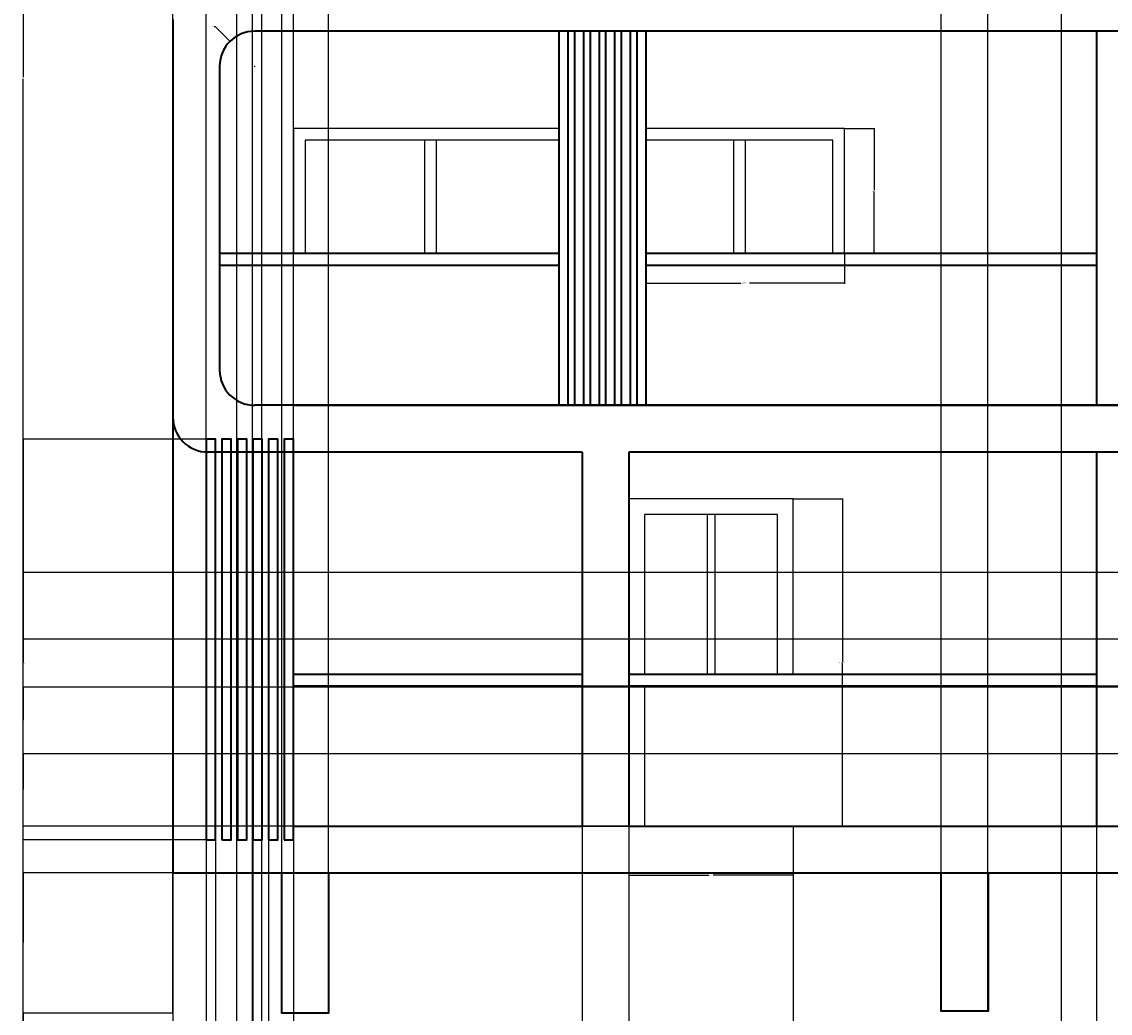
# Model space of a CAD drawing. Units: inches. Extents: x -15 to 605, y -220 to 570.
# Tile 2 of 10: x -15 to 265, y -32 to 222. Entities that reach past the tile are written whole.
import ezdxf

# ---------------------------------------------------------------- set-up
doc = ezdxf.new("R2010")
doc.units = ezdxf.units.IN
doc.header["$MEASUREMENT"] = 0
for name, color, linetype, lineweight in [('A-ANNO-DIMS', 2, 'Continuous', 18), ('A-COLS', 7, 'Continuous', 35), ('A-DOOR', 4, 'Continuous', 25), ('A-ELEV', 7, 'Continuous', 35), ('A-GLAZ', 4, 'Continuous', 25)]:
    doc.layers.add(name, color=color, linetype=linetype, lineweight=lineweight)
doc.styles.get("Standard").update_dxf_attribs({"font": 'arial.ttf'})
doc.dimstyles.get("Standard").update_dxf_attribs({"dimtxt": 0.18, "dimasz": 0.18, "dimexe": 0.18, "dimexo": 0.0625, "dimgap": 0.09, "dimtad": 0, "dimtih": 1, "dimtoh": 1, "dimdec": 4, "dimzin": 0, "dimdsep": 46, "dimtxsty": 'Standard', "dimcen": 0.09, "dimadec": 0, "dimazin": 0, "dimtfac": 1, "dimtdec": 4, "dimtofl": 0, "dimtmove": 0, "dimatfit": 3, "dimfxl": 1, "dimtolj": 1, "dimtzin": 0, "dimarcsym": 0})

# ---------------------------------------------------------------- blocks, each defined once
blk = doc.blocks.new('DOOR-ELEV')
for p, q in [((20.09, 80), (20.09, 39)), ((22.09, 80), (22.09, 39))]:
    blk.add_line(p, q)
for points in [[(42.18, 39), (42.18, 84), (0, 84), (0, 0), (42.18, 0)], [(38.18, 39), (38.18, 80), (4, 80), (4, 39)], [(4, 36), (4, 0)]]:
    blk.add_lwpolyline(points)
blk = doc.blocks.new('WIN-ELEV')
for p, q in [((22.41, 29.07), (22.41, 0)), ((25.41, 29.07), (25.41, 0))]:
    blk.add_line(p, q)
for points in [[(50.87, 0), (50.87, 32.07), (0, 32.07)], [(47.87, 0), (47.87, 29.07), (0, 29.07)]]:
    blk.add_lwpolyline(points)
blk = doc.blocks.new('*D3')
at = {"layer": 'A-ANNO-DIMS', "color": 0, "lineweight": -2, "transparency": 16777216}
for p, q in [((183.23, 99.82), (195.95, 99.82)), ((195.77, 99.64), (195.77, 58)), ((195.77, 16), (195.77, 57.64)), ((183.23, 15.82), (195.95, 15.82))]:
    blk.add_line(p, q, dxfattribs=at)
at = {"layer": 'A-ANNO-DIMS', "color": 0, "transparency": 16777216}
for points in [[(195.74, 99.64), (195.8, 99.64), (195.77, 99.82)], [(195.74, 16), (195.8, 16), (195.77, 15.82)]]:
    blk.add_solid(points, dxfattribs=at)
at = {"layer": 'Defpoints', "color": 0, "transparency": 16777216}
for p in [(183.17, 99.82), (195.77, 99.82), (183.17, 15.82)]:
    blk.add_point(p, dxfattribs=at)
at = {"layer": 'A-ANNO-DIMS', "color": 0, "transparency": 16777216, "insert": (195.77, 57.82), "char_height": 0.18, "attachment_point": 5}
blk.add_mtext('\\A1;DOOR 84 TYP.', dxfattribs=at)
blk = doc.blocks.new('*D4')
at = {"layer": 'A-ANNO-DIMS', "color": 0, "lineweight": -2, "transparency": 16777216}
for p, q in [((140.99, 15.76), (140.99, 3.04)), ((183.17, 15.76), (183.17, 3.04)), ((141.17, 3.22), (161.55, 3.22)), ((182.99, 3.22), (162.61, 3.22))]:
    blk.add_line(p, q, dxfattribs=at)
at = {"layer": 'A-ANNO-DIMS', "color": 0, "transparency": 16777216}
for points in [[(141.17, 3.25), (141.17, 3.19), (140.99, 3.22)], [(182.99, 3.25), (182.99, 3.19), (183.17, 3.22)]]:
    blk.add_solid(points, dxfattribs=at)
at = {"layer": 'Defpoints', "color": 0, "transparency": 16777216}
for p in [(140.99, 15.82), (183.17, 15.82), (183.17, 3.22)]:
    blk.add_point(p, dxfattribs=at)
at = {"layer": 'A-ANNO-DIMS', "color": 0, "transparency": 16777216, "insert": (162.08, 3.22), "char_height": 0.18, "attachment_point": 5}
blk.add_mtext('\\A1;42 TYP.', dxfattribs=at)
blk = doc.blocks.new('*D5')
at = {"layer": 'A-ANNO-DIMS', "color": 0, "lineweight": -2, "transparency": 16777216}
for p, q in [((145.43, 162.76), (145.43, 155.01)), ((196.29, 162.76), (196.29, 155.01)), ((145.61, 155.19), (169.74, 155.19)), ((196.11, 155.19), (171.98, 155.19))]:
    blk.add_line(p, q, dxfattribs=at)
at = {"layer": 'A-ANNO-DIMS', "color": 0, "transparency": 16777216}
for points in [[(145.61, 155.22), (145.61, 155.16), (145.43, 155.19)], [(196.11, 155.22), (196.11, 155.16), (196.29, 155.19)]]:
    blk.add_solid(points, dxfattribs=at)
at = {"layer": 'Defpoints', "color": 0, "transparency": 16777216}
for p in [(145.43, 162.82), (196.29, 162.82), (196.29, 155.19)]:
    blk.add_point(p, dxfattribs=at)
at = {"layer": 'A-ANNO-DIMS', "color": 0, "transparency": 16777216, "insert": (170.86, 155.19), "char_height": 0.18, "attachment_point": 5}
blk.add_mtext('\\A1;WINDOW 51 TYP.', dxfattribs=at)
blk = doc.blocks.new('*D6')
at = {"layer": 'A-ANNO-DIMS', "color": 0, "lineweight": -2, "transparency": 16777216}
for p, q in [((196.36, 194.89), (204.1, 194.89)), ((203.92, 194.71), (203.92, 179.04)), ((203.92, 163), (203.92, 178.67)), ((196.36, 162.82), (204.1, 162.82))]:
    blk.add_line(p, q, dxfattribs=at)
at = {"layer": 'A-ANNO-DIMS', "color": 0, "transparency": 16777216}
for points in [[(203.89, 194.71), (203.95, 194.71), (203.92, 194.89)], [(203.89, 163), (203.95, 163), (203.92, 162.82)]]:
    blk.add_solid(points, dxfattribs=at)
at = {"layer": 'Defpoints', "color": 0, "transparency": 16777216}
for p in [(196.29, 194.89), (203.92, 194.89), (196.29, 162.82)]:
    blk.add_point(p, dxfattribs=at)
at = {"layer": 'A-ANNO-DIMS', "color": 0, "transparency": 16777216, "insert": (203.92, 178.85), "char_height": 0.18, "attachment_point": 5}
blk.add_mtext('\\A1;32 TYP.', dxfattribs=at)
blk = doc.blocks.new('*D7')
at = {"layer": 'A-ANNO-DIMS', "color": 0, "lineweight": -2, "transparency": 16777216}
for p, q in [((23.99, 3.76), (23.99, -154.76)), ((566.72, -116.24), (566.72, -154.76)), ((24.17, -154.58), (294.96, -154.58)), ((566.54, -154.58), (295.75, -154.58))]:
    blk.add_line(p, q, dxfattribs=at)
at = {"layer": 'A-ANNO-DIMS', "color": 0, "transparency": 16777216}
for points in [[(24.17, -154.55), (24.17, -154.61), (23.99, -154.58)], [(566.54, -154.55), (566.54, -154.61), (566.72, -154.58)]]:
    blk.add_solid(points, dxfattribs=at)
at = {"layer": 'Defpoints', "color": 0, "transparency": 16777216}
for p in [(23.99, 3.82), (566.72, -116.18), (566.72, -154.58)]:
    blk.add_point(p, dxfattribs=at)
at = {"layer": 'A-ANNO-DIMS', "color": 0, "transparency": 16777216, "insert": (295.35, -154.58), "char_height": 0.18, "attachment_point": 5}
blk.add_mtext('\\A1;542.7', dxfattribs=at)
blk = doc.blocks.new('*D8')
at = {"layer": 'A-ANNO-DIMS', "color": 0, "lineweight": -2, "transparency": 16777216}
for p, q in [((23.99, 3.88), (23.99, 570.4)), ((24.17, 570.22), (263.7, 570.22)), ((503.81, 570.22), (264.28, 570.22)), ((503.99, 531.88), (503.99, 570.4))]:
    blk.add_line(p, q, dxfattribs=at)
at = {"layer": 'A-ANNO-DIMS', "color": 0, "transparency": 16777216}
for points in [[(24.17, 570.25), (24.17, 570.19), (23.99, 570.22)], [(503.81, 570.25), (503.81, 570.19), (503.99, 570.22)]]:
    blk.add_solid(points, dxfattribs=at)
at = {"layer": 'Defpoints', "color": 0, "transparency": 16777216}
for p in [(503.99, 570.22), (503.99, 531.82), (23.99, 3.82)]:
    blk.add_point(p, dxfattribs=at)
at = {"layer": 'A-ANNO-DIMS', "color": 0, "transparency": 16777216, "insert": (263.99, 570.22), "char_height": 0.18, "attachment_point": 5}
blk.add_mtext('\\A1;480', dxfattribs=at)
blk = doc.blocks.new('*D9')
at = {"layer": 'A-ANNO-DIMS', "color": 0, "lineweight": -2, "transparency": 16777216}
for p, q in [((503.92, 531.82), (-14.59, 531.82)), ((-14.41, 531.64), (-14.41, 208)), ((-14.41, -116), (-14.41, 207.64)), ((23.92, -116.18), (-14.59, -116.18))]:
    blk.add_line(p, q, dxfattribs=at)
at = {"layer": 'A-ANNO-DIMS', "color": 0, "transparency": 16777216}
for points in [[(-14.44, 531.64), (-14.38, 531.64), (-14.41, 531.82)], [(-14.44, -116), (-14.38, -116), (-14.41, -116.18)]]:
    blk.add_solid(points, dxfattribs=at)
at = {"layer": 'Defpoints', "color": 0, "transparency": 16777216}
for p in [(-14.41, 531.82), (503.99, 531.82), (23.99, -116.18)]:
    blk.add_point(p, dxfattribs=at)
at = {"layer": 'A-ANNO-DIMS', "color": 0, "transparency": 16777216, "insert": (-14.41, 207.82), "char_height": 0.18, "attachment_point": 5}
blk.add_mtext('\\A1;648', dxfattribs=at)
blk = doc.blocks.new('*D18')
at = {"layer": 'A-ANNO-DIMS', "color": 0, "lineweight": -2, "transparency": 16777216}
for p, q in [((23.99, 3.88), (23.99, 570.4)), ((24.17, 570.22), (143.44, 570.22)), ((263.64, 570.22), (144.37, 570.22)), ((263.82, 447.88), (263.82, 570.4))]:
    blk.add_line(p, q, dxfattribs=at)
at = {"layer": 'A-ANNO-DIMS', "color": 0, "transparency": 16777216}
for points in [[(24.17, 570.25), (24.17, 570.19), (23.99, 570.22)], [(263.64, 570.25), (263.64, 570.19), (263.82, 570.22)]]:
    blk.add_solid(points, dxfattribs=at)
at = {"layer": 'Defpoints', "color": 0, "transparency": 16777216}
for p in [(263.82, 570.22), (263.82, 447.82), (23.99, 3.82)]:
    blk.add_point(p, dxfattribs=at)
at = {"layer": 'A-ANNO-DIMS', "color": 0, "transparency": 16777216, "insert": (143.9, 570.22), "char_height": 0.18, "attachment_point": 5}
blk.add_mtext('\\A1;239.83', dxfattribs=at)
blk = doc.blocks.new('*D21')
at = {"layer": 'A-ANNO-DIMS', "color": 0, "lineweight": -2, "transparency": 16777216}
for p, q in [((23.92, 3.82), (-14.59, 3.82)), ((-14.41, 3.64), (-14.41, -14)), ((-14.41, -32), (-14.41, -14.36)), ((23.92, -32.18), (-14.59, -32.18))]:
    blk.add_line(p, q, dxfattribs=at)
at = {"layer": 'A-ANNO-DIMS', "color": 0, "transparency": 16777216}
for points in [[(-14.44, 3.64), (-14.38, 3.64), (-14.41, 3.82)], [(-14.44, -32), (-14.38, -32), (-14.41, -32.18)]]:
    blk.add_solid(points, dxfattribs=at)
at = {"layer": 'Defpoints', "color": 0, "transparency": 16777216}
for p in [(-14.41, 3.82), (23.99, 3.82), (23.99, -32.18)]:
    blk.add_point(p, dxfattribs=at)
at = {"layer": 'A-ANNO-DIMS', "color": 0, "transparency": 16777216, "insert": (-14.41, -14.18), "char_height": 0.18, "attachment_point": 5}
blk.add_mtext('\\A1;36', dxfattribs=at)
blk = doc.blocks.new('*D23')
at = {"layer": 'A-ANNO-DIMS', "color": 0, "lineweight": -2, "transparency": 16777216}
for p, q in [((54.93, 15.76), (54.93, -154.76)), ((23.99, 3.76), (23.99, -154.76)), ((24.17, -154.58), (39, -154.58)), ((54.75, -154.58), (39.92, -154.58))]:
    blk.add_line(p, q, dxfattribs=at)
at = {"layer": 'A-ANNO-DIMS', "color": 0, "transparency": 16777216}
for points in [[(24.17, -154.55), (24.17, -154.61), (23.99, -154.58)], [(54.75, -154.55), (54.75, -154.61), (54.93, -154.58)]]:
    blk.add_solid(points, dxfattribs=at)
at = {"layer": 'Defpoints', "color": 0, "transparency": 16777216}
for p in [(54.93, 15.82), (23.99, 3.82), (54.93, -154.58)]:
    blk.add_point(p, dxfattribs=at)
at = {"layer": 'A-ANNO-DIMS', "color": 0, "transparency": 16777216, "insert": (39.46, -154.58), "char_height": 0.18, "attachment_point": 5}
blk.add_mtext('\\A1;30.946', dxfattribs=at)
blk = doc.blocks.new('*D24')
at = {"layer": 'A-ANNO-DIMS', "color": 0, "lineweight": -2, "transparency": 16777216}
for p, q in [((54.93, 15.76), (54.93, -154.76)), ((128.99, 15.76), (128.99, -154.76)), ((55.11, -154.58), (91.57, -154.58)), ((128.81, -154.58), (92.35, -154.58))]:
    blk.add_line(p, q, dxfattribs=at)
at = {"layer": 'A-ANNO-DIMS', "color": 0, "transparency": 16777216}
for points in [[(55.11, -154.55), (55.11, -154.61), (54.93, -154.58)], [(128.81, -154.55), (128.81, -154.61), (128.99, -154.58)]]:
    blk.add_solid(points, dxfattribs=at)
at = {"layer": 'Defpoints', "color": 0, "transparency": 16777216}
for p in [(54.93, 15.82), (128.99, 15.82), (128.99, -154.58)]:
    blk.add_point(p, dxfattribs=at)
at = {"layer": 'A-ANNO-DIMS', "color": 0, "transparency": 16777216, "insert": (91.96, -154.58), "char_height": 0.18, "attachment_point": 5}
blk.add_mtext('\\A1;74.05', dxfattribs=at)
blk = doc.blocks.new('*D25')
at = {"layer": 'A-ANNO-DIMS', "color": 0, "lineweight": -2, "transparency": 16777216}
for p, q in [((128.99, 15.76), (128.99, -154.76)), ((140.99, 15.76), (140.99, -154.76)), ((129.17, -154.58), (134.78, -154.58)), ((140.81, -154.58), (135.2, -154.58))]:
    blk.add_line(p, q, dxfattribs=at)
at = {"layer": 'A-ANNO-DIMS', "color": 0, "transparency": 16777216}
for points in [[(129.17, -154.55), (129.17, -154.61), (128.99, -154.58)], [(140.81, -154.55), (140.81, -154.61), (140.99, -154.58)]]:
    blk.add_solid(points, dxfattribs=at)
at = {"layer": 'Defpoints', "color": 0, "transparency": 16777216}
for p in [(128.99, 15.82), (140.99, 15.82), (140.99, -154.58)]:
    blk.add_point(p, dxfattribs=at)
at = {"layer": 'A-ANNO-DIMS', "color": 0, "transparency": 16777216, "insert": (134.99, -154.58), "char_height": 0.18, "attachment_point": 5}
blk.add_mtext('\\A1;12', dxfattribs=at)
blk = doc.blocks.new('*D26')
at = {"layer": 'A-ANNO-DIMS', "color": 0, "lineweight": -2, "transparency": 16777216}
for p, q in [((140.99, 15.76), (140.99, -154.76)), ((183.17, 15.76), (183.17, -154.76)), ((141.17, -154.58), (161.68, -154.58)), ((182.99, -154.58), (162.48, -154.58))]:
    blk.add_line(p, q, dxfattribs=at)
at = {"layer": 'A-ANNO-DIMS', "color": 0, "transparency": 16777216}
for points in [[(141.17, -154.55), (141.17, -154.61), (140.99, -154.58)], [(182.99, -154.55), (182.99, -154.61), (183.17, -154.58)]]:
    blk.add_solid(points, dxfattribs=at)
at = {"layer": 'Defpoints', "color": 0, "transparency": 16777216}
for p in [(140.99, 15.82), (183.17, 15.82), (183.17, -154.58)]:
    blk.add_point(p, dxfattribs=at)
at = {"layer": 'A-ANNO-DIMS', "color": 0, "transparency": 16777216, "insert": (162.08, -154.58), "char_height": 0.18, "attachment_point": 5}
blk.add_mtext('\\A1;42.18', dxfattribs=at)
blk = doc.blocks.new('*D27')
at = {"layer": 'A-ANNO-DIMS', "color": 0, "lineweight": -2, "transparency": 16777216}
for p, q in [((183.17, 15.76), (183.17, -154.76)), ((260.99, 15.76), (260.99, -154.76)), ((183.35, -154.58), (221.69, -154.58)), ((260.81, -154.58), (222.47, -154.58))]:
    blk.add_line(p, q, dxfattribs=at)
at = {"layer": 'A-ANNO-DIMS', "color": 0, "transparency": 16777216}
for points in [[(183.35, -154.55), (183.35, -154.61), (183.17, -154.58)], [(260.81, -154.55), (260.81, -154.61), (260.99, -154.58)]]:
    blk.add_solid(points, dxfattribs=at)
at = {"layer": 'Defpoints', "color": 0, "transparency": 16777216}
for p in [(183.17, 15.82), (260.99, 15.82), (260.99, -154.58)]:
    blk.add_point(p, dxfattribs=at)
at = {"layer": 'A-ANNO-DIMS', "color": 0, "transparency": 16777216, "insert": (222.08, -154.58), "char_height": 0.18, "attachment_point": 5}
blk.add_mtext('\\A1;77.82', dxfattribs=at)
blk = doc.blocks.new('*D28')
at = {"layer": 'A-ANNO-DIMS', "color": 0, "lineweight": -2, "transparency": 16777216}
for p, q in [((260.99, 15.76), (260.99, -154.76)), ((272.99, 15.76), (272.99, -154.76)), ((261.17, -154.58), (266.78, -154.58)), ((272.81, -154.58), (267.2, -154.58))]:
    blk.add_line(p, q, dxfattribs=at)
at = {"layer": 'A-ANNO-DIMS', "color": 0, "transparency": 16777216}
for points in [[(261.17, -154.55), (261.17, -154.61), (260.99, -154.58)], [(272.81, -154.55), (272.81, -154.61), (272.99, -154.58)]]:
    blk.add_solid(points, dxfattribs=at)
at = {"layer": 'Defpoints', "color": 0, "transparency": 16777216}
for p in [(260.99, 15.82), (272.99, 15.82), (272.99, -154.58)]:
    blk.add_point(p, dxfattribs=at)
at = {"layer": 'A-ANNO-DIMS', "color": 0, "transparency": 16777216, "insert": (266.99, -154.58), "char_height": 0.18, "attachment_point": 5}
blk.add_mtext('\\A1;12', dxfattribs=at)
blk = doc.blocks.new('*D33')
at = {"layer": 'A-ANNO-DIMS', "color": 0, "lineweight": -2, "transparency": 16777216}
for p, q in [((491.92, 34.38), (-14.59, 34.38)), ((-14.41, 34.2), (-14.41, 25.28)), ((-14.41, 16), (-14.41, 24.92)), ((491.92, 15.82), (-14.59, 15.82))]:
    blk.add_line(p, q, dxfattribs=at)
at = {"layer": 'A-ANNO-DIMS', "color": 0, "transparency": 16777216}
for points in [[(-14.44, 34.2), (-14.38, 34.2), (-14.41, 34.38)], [(-14.44, 16), (-14.38, 16), (-14.41, 15.82)]]:
    blk.add_solid(points, dxfattribs=at)
at = {"layer": 'Defpoints', "color": 0, "transparency": 16777216}
for p in [(-14.41, 34.38), (491.99, 34.38), (491.99, 15.82)]:
    blk.add_point(p, dxfattribs=at)
at = {"layer": 'A-ANNO-DIMS', "color": 0, "transparency": 16777216, "insert": (-14.41, 25.1), "char_height": 0.18, "attachment_point": 5}
blk.add_mtext('\\A1;18.557', dxfattribs=at)
blk = doc.blocks.new('*D34')
at = {"layer": 'A-ANNO-DIMS', "color": 0, "lineweight": -2, "transparency": 16777216}
for p, q in [((491.92, 51.48), (-14.59, 51.48)), ((-14.41, 51.3), (-14.41, 43.11)), ((-14.41, 34.56), (-14.41, 42.75)), ((491.92, 34.38), (-14.59, 34.38))]:
    blk.add_line(p, q, dxfattribs=at)
at = {"layer": 'A-ANNO-DIMS', "color": 0, "transparency": 16777216}
for points in [[(-14.44, 51.3), (-14.38, 51.3), (-14.41, 51.48)], [(-14.44, 34.56), (-14.38, 34.56), (-14.41, 34.38)]]:
    blk.add_solid(points, dxfattribs=at)
at = {"layer": 'Defpoints', "color": 0, "transparency": 16777216}
for p in [(-14.41, 51.48), (491.99, 51.48), (491.99, 34.38)]:
    blk.add_point(p, dxfattribs=at)
at = {"layer": 'A-ANNO-DIMS', "color": 0, "transparency": 16777216, "insert": (-14.41, 42.93), "char_height": 0.18, "attachment_point": 5}
blk.add_mtext('\\A1;17.1', dxfattribs=at)
blk = doc.blocks.new('*D35')
at = {"layer": 'A-ANNO-DIMS', "color": 0, "lineweight": -2, "transparency": 16777216}
for p, q in [((491.92, 63.82), (-14.59, 63.82)), ((-14.41, 63.64), (-14.41, 57.83)), ((-14.41, 51.66), (-14.41, 57.47)), ((491.92, 51.48), (-14.59, 51.48))]:
    blk.add_line(p, q, dxfattribs=at)
at = {"layer": 'A-ANNO-DIMS', "color": 0, "transparency": 16777216}
for points in [[(-14.44, 63.64), (-14.38, 63.64), (-14.41, 63.82)], [(-14.44, 51.66), (-14.38, 51.66), (-14.41, 51.48)]]:
    blk.add_solid(points, dxfattribs=at)
at = {"layer": 'Defpoints', "color": 0, "transparency": 16777216}
for p in [(-14.41, 63.82), (491.99, 63.82), (491.99, 51.48)]:
    blk.add_point(p, dxfattribs=at)
at = {"layer": 'A-ANNO-DIMS', "color": 0, "transparency": 16777216, "insert": (-14.41, 57.65), "char_height": 0.18, "attachment_point": 5}
blk.add_mtext('\\A1;12.342', dxfattribs=at)
blk = doc.blocks.new('*D36')
at = {"layer": 'A-ANNO-DIMS', "color": 0, "lineweight": -2, "transparency": 16777216}
for p, q in [((491.92, 80.92), (-14.59, 80.92)), ((-14.41, 80.74), (-14.41, 72.55)), ((-14.41, 64), (-14.41, 72.19)), ((491.92, 63.82), (-14.59, 63.82))]:
    blk.add_line(p, q, dxfattribs=at)
at = {"layer": 'A-ANNO-DIMS', "color": 0, "transparency": 16777216}
for points in [[(-14.44, 80.74), (-14.38, 80.74), (-14.41, 80.92)], [(-14.44, 64), (-14.38, 64), (-14.41, 63.82)]]:
    blk.add_solid(points, dxfattribs=at)
at = {"layer": 'Defpoints', "color": 0, "transparency": 16777216}
for p in [(-14.41, 80.92), (491.99, 80.92), (491.99, 63.82)]:
    blk.add_point(p, dxfattribs=at)
at = {"layer": 'A-ANNO-DIMS', "color": 0, "transparency": 16777216, "insert": (-14.41, 72.37), "char_height": 0.18, "attachment_point": 5}
blk.add_mtext('\\A1;17.1', dxfattribs=at)
blk = doc.blocks.new('*D37')
at = {"layer": 'A-ANNO-DIMS', "color": 0, "lineweight": -2, "transparency": 16777216}
for p, q in [((129.05, 51.82), (605.3, 51.82)), ((605.12, 51.64), (605.12, 34)), ((605.12, 16), (605.12, 33.64)), ((129.05, 15.82), (605.3, 15.82))]:
    blk.add_line(p, q, dxfattribs=at)
at = {"layer": 'A-ANNO-DIMS', "color": 0, "transparency": 16777216}
for points in [[(605.09, 51.64), (605.15, 51.64), (605.12, 51.82)], [(605.09, 16), (605.15, 16), (605.12, 15.82)]]:
    blk.add_solid(points, dxfattribs=at)
at = {"layer": 'Defpoints', "color": 0, "transparency": 16777216}
for p in [(128.99, 51.82), (605.12, 51.82), (128.99, 15.82)]:
    blk.add_point(p, dxfattribs=at)
at = {"layer": 'A-ANNO-DIMS', "color": 0, "transparency": 16777216, "insert": (605.12, 33.82), "char_height": 0.18, "attachment_point": 5}
blk.add_mtext('\\A1;36', dxfattribs=at)
blk = doc.blocks.new('*D38')
at = {"layer": 'A-ANNO-DIMS', "color": 0, "lineweight": -2, "transparency": 16777216}
for p, q in [((32.47, 115.12), (-14.59, 115.12)), ((-14.41, 114.94), (-14.41, 63.88)), ((-14.41, 12.46), (-14.41, 63.52)), ((32.47, 12.28), (-14.59, 12.28))]:
    blk.add_line(p, q, dxfattribs=at)
at = {"layer": 'A-ANNO-DIMS', "color": 0, "transparency": 16777216}
for points in [[(-14.44, 114.94), (-14.38, 114.94), (-14.41, 115.12)], [(-14.44, 12.46), (-14.38, 12.46), (-14.41, 12.28)]]:
    blk.add_solid(points, dxfattribs=at)
at = {"layer": 'Defpoints', "color": 0, "transparency": 16777216}
for p in [(-14.41, 115.12), (32.53, 115.12), (32.53, 12.28)]:
    blk.add_point(p, dxfattribs=at)
at = {"layer": 'A-ANNO-DIMS', "color": 0, "transparency": 16777216, "insert": (-14.41, 63.7), "char_height": 0.18, "attachment_point": 5}
blk.add_mtext('\\A1;102.84', dxfattribs=at)
blk = doc.blocks.new('*D52')
at = {"layer": 'A-ANNO-DIMS', "color": 0, "lineweight": -2, "transparency": 16777216}
for p, q in [((23.99, -32.12), (23.99, 570.4)), ((24.17, 570.22), (37.55, 570.22)), ((51.73, 570.22), (38.34, 570.22)), ((51.91, -32.12), (51.91, 570.4))]:
    blk.add_line(p, q, dxfattribs=at)
at = {"layer": 'A-ANNO-DIMS', "color": 0, "transparency": 16777216}
for points in [[(24.17, 570.25), (24.17, 570.19), (23.99, 570.22)], [(51.73, 570.25), (51.73, 570.19), (51.91, 570.22)]]:
    blk.add_solid(points, dxfattribs=at)
at = {"layer": 'Defpoints', "color": 0, "transparency": 16777216}
for p in [(51.91, 570.22), (23.99, -32.18), (51.91, -32.18)]:
    blk.add_point(p, dxfattribs=at)
at = {"layer": 'A-ANNO-DIMS', "color": 0, "transparency": 16777216, "insert": (37.95, 570.22), "char_height": 0.18, "attachment_point": 5}
blk.add_mtext('\\A1;27.92', dxfattribs=at)
blk = doc.blocks.new('*D53')
at = {"layer": 'A-ANNO-DIMS', "color": 0, "lineweight": -2, "transparency": 16777216}
for p, q in [((51.91, -32.12), (51.91, 570.4)), ((52.09, 570.22), (57.7, 570.22)), ((63.73, 570.22), (58.12, 570.22)), ((63.91, -32.12), (63.91, 570.4))]:
    blk.add_line(p, q, dxfattribs=at)
at = {"layer": 'A-ANNO-DIMS', "color": 0, "transparency": 16777216}
for points in [[(52.09, 570.25), (52.09, 570.19), (51.91, 570.22)], [(63.73, 570.25), (63.73, 570.19), (63.91, 570.22)]]:
    blk.add_solid(points, dxfattribs=at)
at = {"layer": 'Defpoints', "color": 0, "transparency": 16777216}
for p in [(63.91, 570.22), (51.91, -32.18), (63.91, -32.18)]:
    blk.add_point(p, dxfattribs=at)
at = {"layer": 'A-ANNO-DIMS', "color": 0, "transparency": 16777216, "insert": (57.91, 570.22), "char_height": 0.18, "attachment_point": 5}
blk.add_mtext('\\A1;12', dxfattribs=at)
blk = doc.blocks.new('*D54')
at = {"layer": 'A-ANNO-DIMS', "color": 0, "lineweight": -2, "transparency": 16777216}
for p, q in [((63.91, -32.12), (63.91, 570.4)), ((64.09, 570.22), (142.07, 570.22)), ((220.96, 570.22), (142.98, 570.22)), ((221.14, -31.58), (221.14, 570.4))]:
    blk.add_line(p, q, dxfattribs=at)
at = {"layer": 'A-ANNO-DIMS', "color": 0, "transparency": 16777216}
for points in [[(64.09, 570.25), (64.09, 570.19), (63.91, 570.22)], [(220.96, 570.25), (220.96, 570.19), (221.14, 570.22)]]:
    blk.add_solid(points, dxfattribs=at)
at = {"layer": 'Defpoints', "color": 0, "transparency": 16777216}
for p in [(221.14, 570.22), (63.91, -32.18), (221.14, -31.64)]:
    blk.add_point(p, dxfattribs=at)
at = {"layer": 'A-ANNO-DIMS', "color": 0, "transparency": 16777216, "insert": (142.53, 570.22), "char_height": 0.18, "attachment_point": 5}
blk.add_mtext('\\A1;157.24', dxfattribs=at)
blk = doc.blocks.new('*D55')
at = {"layer": 'A-ANNO-DIMS', "color": 0, "lineweight": -2, "transparency": 16777216}
for p, q in [((221.14, -31.58), (221.14, 570.4)), ((221.32, 570.22), (226.93, 570.22)), ((232.96, 570.22), (227.35, 570.22)), ((233.14, -31.58), (233.14, 570.4))]:
    blk.add_line(p, q, dxfattribs=at)
at = {"layer": 'A-ANNO-DIMS', "color": 0, "transparency": 16777216}
for points in [[(221.32, 570.25), (221.32, 570.19), (221.14, 570.22)], [(232.96, 570.25), (232.96, 570.19), (233.14, 570.22)]]:
    blk.add_solid(points, dxfattribs=at)
at = {"layer": 'Defpoints', "color": 0, "transparency": 16777216}
for p in [(233.14, 570.22), (221.14, -31.64), (233.14, -31.64)]:
    blk.add_point(p, dxfattribs=at)
at = {"layer": 'A-ANNO-DIMS', "color": 0, "transparency": 16777216, "insert": (227.14, 570.22), "char_height": 0.18, "attachment_point": 5}
blk.add_mtext('\\A1;12', dxfattribs=at)
blk = doc.blocks.new('*D56')
at = {"layer": 'A-ANNO-DIMS', "color": 0, "lineweight": -2, "transparency": 16777216}
for p, q in [((233.14, -31.58), (233.14, 570.4)), ((233.32, 570.22), (298.47, 570.22)), ((364.53, 570.22), (299.38, 570.22)), ((364.71, -56.12), (364.71, 570.4))]:
    blk.add_line(p, q, dxfattribs=at)
at = {"layer": 'A-ANNO-DIMS', "color": 0, "transparency": 16777216}
for points in [[(233.32, 570.25), (233.32, 570.19), (233.14, 570.22)], [(364.53, 570.25), (364.53, 570.19), (364.71, 570.22)]]:
    blk.add_solid(points, dxfattribs=at)
at = {"layer": 'Defpoints', "color": 0, "transparency": 16777216}
for p in [(364.71, 570.22), (233.14, -31.64), (364.71, -56.18)]:
    blk.add_point(p, dxfattribs=at)
at = {"layer": 'A-ANNO-DIMS', "color": 0, "transparency": 16777216, "insert": (298.93, 570.22), "char_height": 0.18, "attachment_point": 5}
blk.add_mtext('\\A1;131.56', dxfattribs=at)
blk = doc.blocks.new('*D64')
at = {"layer": 'A-ANNO-DIMS', "color": 0, "lineweight": -2, "transparency": 16777216}
for p, q in [((23.92, -32.18), (-14.59, -32.18)), ((-14.41, -32.36), (-14.41, -74)), ((-14.41, -116), (-14.41, -74.36)), ((23.92, -116.18), (-14.59, -116.18))]:
    blk.add_line(p, q, dxfattribs=at)
at = {"layer": 'A-ANNO-DIMS', "color": 0, "transparency": 16777216}
for points in [[(-14.44, -32.36), (-14.38, -32.36), (-14.41, -32.18)], [(-14.44, -116), (-14.38, -116), (-14.41, -116.18)]]:
    blk.add_solid(points, dxfattribs=at)
at = {"layer": 'Defpoints', "color": 0, "transparency": 16777216}
for p in [(-14.41, -32.18), (23.99, -32.18), (23.99, -116.18)]:
    blk.add_point(p, dxfattribs=at)
at = {"layer": 'A-ANNO-DIMS', "color": 0, "transparency": 16777216, "insert": (-14.41, -74.18), "char_height": 0.18, "attachment_point": 5}
blk.add_mtext('\\A1;84', dxfattribs=at)
blk = doc.blocks.new('*D99')
at = {"layer": 'A-ANNO-DIMS', "color": 0, "lineweight": -2, "transparency": 16777216}
for p, q in [((34.62, 221), (34.8, 221)), ((34.8, 221), (38.5, 217.31)), ((44.9, 210.82), (45.08, 210.82)), ((44.99, 210.73), (44.99, 210.91))]:
    blk.add_line(p, q, dxfattribs=at)
at = {"layer": 'A-ANNO-DIMS', "color": 0, "transparency": 16777216}
blk.add_solid([(38.52, 217.33), (38.47, 217.29), (38.62, 217.18)], dxfattribs=at)
at = {"layer": 'Defpoints', "color": 0, "transparency": 16777216}
for p in [(38.62, 217.18), (44.99, 210.82)]:
    blk.add_point(p, dxfattribs=at)
at = {"layer": 'A-ANNO-DIMS', "color": 0, "transparency": 16777216, "insert": (34.2, 221), "char_height": 0.18, "attachment_point": 5}
blk.add_mtext('\\A1;8X R9', dxfattribs=at)
blk = doc.blocks.new('*D104')
at = {"layer": 'A-ANNO-DIMS', "color": 0, "lineweight": -2, "transparency": 16777216}
for p, q in [((251.99, -56.12), (251.99, 570.4)), ((252.17, 570.22), (267.39, 570.22)), ((283.41, 570.22), (268.18, 570.22)), ((283.59, -84.79), (283.59, 570.4))]:
    blk.add_line(p, q, dxfattribs=at)
at = {"layer": 'A-ANNO-DIMS', "color": 0, "transparency": 16777216}
for points in [[(252.17, 570.25), (252.17, 570.19), (251.99, 570.22)], [(283.41, 570.25), (283.41, 570.19), (283.59, 570.22)]]:
    blk.add_solid(points, dxfattribs=at)
at = {"layer": 'Defpoints', "color": 0, "transparency": 16777216}
for p in [(283.59, 570.22), (251.99, -56.18), (283.59, -84.86)]:
    blk.add_point(p, dxfattribs=at)
at = {"layer": 'A-ANNO-DIMS', "color": 0, "transparency": 16777216, "insert": (267.79, 570.22), "char_height": 0.18, "attachment_point": 5}
blk.add_mtext('\\A1;31.60', dxfattribs=at)
blk = doc.blocks.new('*D110')
at = {"layer": 'A-ANNO-DIMS', "color": 0, "lineweight": -2, "transparency": 16777216}
for p, q in [((32.53, 115.18), (32.53, 570.4)), ((32.71, 570.22), (43.34, 570.22)), ((54.75, 570.22), (44.13, 570.22)), ((54.93, 115.18), (54.93, 570.4))]:
    blk.add_line(p, q, dxfattribs=at)
at = {"layer": 'A-ANNO-DIMS', "color": 0, "transparency": 16777216}
for points in [[(32.71, 570.25), (32.71, 570.19), (32.53, 570.22)], [(54.75, 570.25), (54.75, 570.19), (54.93, 570.22)]]:
    blk.add_solid(points, dxfattribs=at)
at = {"layer": 'Defpoints', "color": 0, "transparency": 16777216}
for p in [(54.93, 570.22), (32.53, 115.12), (54.93, 115.12)]:
    blk.add_point(p, dxfattribs=at)
at = {"layer": 'A-ANNO-DIMS', "color": 0, "transparency": 16777216, "insert": (43.73, 570.22), "char_height": 0.18, "attachment_point": 5}
blk.add_mtext('\\A1;22.40', dxfattribs=at)
blk = doc.blocks.new('*D111')
at = {"layer": 'A-ANNO-DIMS', "color": 0, "lineweight": -2, "transparency": 16777216}
for p, q in [((32.53, 12.22), (32.53, -154.76)), ((34.93, 12.22), (34.93, -154.76)), ((32.71, -154.58), (33.41, -154.58)), ((34.75, -154.58), (34.06, -154.58))]:
    blk.add_line(p, q, dxfattribs=at)
at = {"layer": 'A-ANNO-DIMS', "color": 0, "transparency": 16777216}
for points in [[(32.71, -154.55), (32.71, -154.61), (32.53, -154.58)], [(34.75, -154.55), (34.75, -154.61), (34.93, -154.58)]]:
    blk.add_solid(points, dxfattribs=at)
at = {"layer": 'Defpoints', "color": 0, "transparency": 16777216}
for p in [(32.53, 12.28), (34.93, 12.28), (34.93, -154.58)]:
    blk.add_point(p, dxfattribs=at)
at = {"layer": 'A-ANNO-DIMS', "color": 0, "transparency": 16777216, "insert": (33.73, -154.58), "char_height": 0.18, "attachment_point": 5}
blk.add_mtext('\\A1;2.40', dxfattribs=at)
blk = doc.blocks.new('*D112')
at = {"layer": 'A-ANNO-DIMS', "color": 0, "lineweight": -2, "transparency": 16777216}
for p, q in [((44.53, 12.22), (44.53, -154.76)), ((48.53, 12.22), (48.53, -154.76)), ((44.71, -154.58), (46.21, -154.58)), ((48.35, -154.58), (46.86, -154.58))]:
    blk.add_line(p, q, dxfattribs=at)
at = {"layer": 'A-ANNO-DIMS', "color": 0, "transparency": 16777216}
for points in [[(44.71, -154.55), (44.71, -154.61), (44.53, -154.58)], [(48.35, -154.55), (48.35, -154.61), (48.53, -154.58)]]:
    blk.add_solid(points, dxfattribs=at)
at = {"layer": 'Defpoints', "color": 0, "transparency": 16777216}
for p in [(44.53, 12.28), (48.53, 12.28), (48.53, -154.58)]:
    blk.add_point(p, dxfattribs=at)
at = {"layer": 'A-ANNO-DIMS', "color": 0, "transparency": 16777216, "insert": (46.53, -154.58), "char_height": 0.18, "attachment_point": 5}
blk.add_mtext('\\A1;4.00', dxfattribs=at)
blk = doc.blocks.new('*D113')
at = {"layer": 'A-ANNO-DIMS', "color": 0, "lineweight": -2, "transparency": 16777216}
for p, q in [((44.35, 231.76), (44.35, -154.76)), ((46.75, 231.76), (46.75, -154.76)), ((44.53, -154.58), (45.23, -154.58)), ((46.57, -154.58), (45.88, -154.58))]:
    blk.add_line(p, q, dxfattribs=at)
at = {"layer": 'A-ANNO-DIMS', "color": 0, "transparency": 16777216}
for points in [[(44.53, -154.55), (44.53, -154.61), (44.35, -154.58)], [(46.57, -154.55), (46.57, -154.61), (46.75, -154.58)]]:
    blk.add_solid(points, dxfattribs=at)
at = {"layer": 'Defpoints', "color": 0, "transparency": 16777216}
for p in [(44.35, 231.82), (46.75, 231.82), (46.75, -154.58)]:
    blk.add_point(p, dxfattribs=at)
at = {"layer": 'A-ANNO-DIMS', "color": 0, "transparency": 16777216, "insert": (45.55, -154.58), "char_height": 0.18, "attachment_point": 5}
blk.add_mtext('\\A1;2.40', dxfattribs=at)
blk = doc.blocks.new('*D114')
at = {"layer": 'A-ANNO-DIMS', "color": 0, "lineweight": -2, "transparency": 16777216}
for p, q in [((40.35, 231.76), (40.35, -154.76)), ((44.35, 231.76), (44.35, -154.76)), ((40.53, -154.58), (42.03, -154.58)), ((44.17, -154.58), (42.68, -154.58))]:
    blk.add_line(p, q, dxfattribs=at)
at = {"layer": 'A-ANNO-DIMS', "color": 0, "transparency": 16777216}
for points in [[(40.53, -154.55), (40.53, -154.61), (40.35, -154.58)], [(44.17, -154.55), (44.17, -154.61), (44.35, -154.58)]]:
    blk.add_solid(points, dxfattribs=at)
at = {"layer": 'Defpoints', "color": 0, "transparency": 16777216}
for p in [(40.35, 231.82), (44.35, 231.82), (44.35, -154.58)]:
    blk.add_point(p, dxfattribs=at)
at = {"layer": 'A-ANNO-DIMS', "color": 0, "transparency": 16777216, "insert": (42.35, -154.58), "char_height": 0.18, "attachment_point": 5}
blk.add_mtext('\\A1;4.00', dxfattribs=at)

msp = doc.modelspace()

# ---------------------------------------------------------------- linework, layer by layer
at = {"layer": 'A-COLS'}
for points in [[(51.9067, 3.8187), (63.9067, 3.8187), (63.9067, -32.1813), (51.9067, -32.1813)], [(221.1439, 3.8187), (233.1439, 3.8187), (233.1439, -31.6396), (221.1439, -31.6396)]]:
    msp.add_lwpolyline(points, close=True, dxfattribs=at)
at = {"layer": 'A-ELEV'}
for p, q in [((373.1921, 219.8187), (44.9872, 219.8187)), ((260.9872, 219.8187), (260.9872, 123.8187)), ((373.1921, 123.8187), (44.9872, 123.8187)), ((54.933, 123.8187), (212.3003, 123.8187)), ((54.933, 123.8187), (196.294, 123.8187)), ((212.3003, 123.8187), (260.9872, 123.8187)), ((260.9872, 123.8187), (373.1921, 123.8187)), ((128.9872, 111.8187), (32.9872, 111.8187)), ((128.9872, 111.8187), (128.9872, 15.8187)), ((140.9872, 111.8187), (140.9872, 15.8187)), ((491.9872, 111.8187), (140.9872, 111.8187)), ((260.9872, 111.8187), (260.9872, 15.8187)), ((54.933, 15.8187), (128.9872, 15.8187)), ((140.9872, 15.8187), (212.3003, 15.8187)), ((212.3003, 15.8187), (260.9872, 15.8187)), ((260.9872, 15.8187), (491.9872, 15.8187))]:
    msp.add_line(p, q, dxfattribs=at)
for points in [[(23.9872, 123.8187), (23.9872, 3.8187), (503.9872, 3.8187), (503.9872, 123.8187), (503.9872, 531.8187)], [(123.0266, 219.8187), (123.0266, 123.8187), (125.4266, 123.8187), (125.4266, 219.8187)], [(127.0267, 219.8187), (127.0267, 123.8187), (129.4268, 123.8187), (129.4268, 219.8187)], [(131.0268, 219.8187), (131.0268, 123.8187), (133.4269, 123.8187), (133.4269, 219.8187)], [(135.0269, 219.8187), (135.0269, 123.8187), (137.427, 123.8187), (137.427, 219.8187)], [(139.027, 219.8187), (139.027, 123.8187), (141.4271, 123.8187), (141.4271, 219.8187)], [(143.0272, 219.8187), (143.0272, 123.8187), (145.4272, 123.8187), (145.4272, 219.8187)], [(35.9872, 162.8187), (74.3396, 162.8187), (123.0266, 162.8187)], [(145.4272, 162.8187), (212.3003, 162.8187), (260.9872, 162.8187)], [(35.9872, 159.8187), (74.3396, 159.8187), (123.0266, 159.8187)], [(145.4272, 159.8187), (212.3003, 159.8187), (260.9872, 159.8187)], [(54.933, 54.8187), (128.9872, 54.8187)], [(140.9872, 54.8187), (212.3003, 54.8187), (260.9872, 54.8187)], [(54.933, 51.8187), (128.9872, 51.8187)], [(140.9872, 51.8187), (212.3003, 51.8187), (260.9872, 51.8187)]]:
    msp.add_lwpolyline(points, dxfattribs=at)
for points in [[(23.9872, 222.8187), (23.9872, 120.8187, 0.41421356), (32.9872, 111.8187)], [(35.9872, 210.8187), (35.9872, 132.8187, 0.41421356), (44.9872, 123.8187)]]:
    msp.add_lwpolyline(points, format="xyb", dxfattribs=at)
for points in [[(32.5323, 12.2791), (34.9324, 12.2791), (34.9324, 115.1203), (32.5323, 115.1203)], [(36.5324, 12.2791), (38.9325, 12.2791), (38.9325, 115.1203), (36.5324, 115.1203)], [(40.5325, 12.2791), (42.9326, 12.2791), (42.9326, 115.1203), (40.5325, 115.1203)], [(44.5327, 12.2791), (46.9327, 12.2791), (46.9327, 115.1203), (44.5327, 115.1203)], [(48.5328, 12.2791), (50.9329, 12.2791), (50.9329, 115.1203), (48.5328, 115.1203)], [(52.5329, 12.2791), (54.933, 12.2791), (54.933, 115.1203), (52.5329, 115.1203)]]:
    msp.add_lwpolyline(points, close=True, dxfattribs=at)
msp.add_arc((44.9872, 210.8187), 9, 90, 180, dxfattribs=at)
at = {"layer": 'A-GLAZ'}
for p, q in [((88.549, 191.8893), (88.549, 162.8187)), ((91.549, 191.8893), (91.549, 162.8187))]:
    msp.add_line(p, q, dxfattribs=at)
for points in [[(123.0266, 194.8893), (54.933, 194.8893), (54.933, 162.8187)], [(123.0266, 191.8893), (57.933, 191.8893), (57.933, 162.8187)]]:
    msp.add_lwpolyline(points, dxfattribs=at)

# ---------------------------------------------------------------- block references
at = {"layer": 'A-DOOR'}
msp.add_blockref('DOOR-ELEV', (140.987, 15.819), dxfattribs=at)
at = {"layer": 'A-GLAZ'}
msp.add_blockref('WIN-ELEV', (145.427, 162.819), dxfattribs=at)

# ---------------------------------------------------------------- dimensions: what is measured, and where the dimension line sits
at = {"layer": 'A-ANNO-DIMS'}
for base, p1, p2, override, picture, middle in [((503.9872, 570.2187), (23.9872, 3.8187), (503.9872, 531.8187), {"dimdec": 0, "dimlfac": 1, "dimrnd": 0, "dimzin": 0, "dimdsep": 46, "dimlunit": 2}, '*D8', (263.9872, 570.2187)), ((263.8163, 570.2187), (23.9872, 3.8187), (263.8163, 447.8187), {"dimdec": 2, "dimlfac": 1, "dimrnd": 0, "dimzin": 0, "dimdsep": 46, "dimlunit": 2}, '*D18', (143.9018, 570.2187)), ((51.9067, 570.2187), (23.9872, -32.1813), (51.9067, -32.1813), {"dimdec": 2, "dimlfac": 1, "dimrnd": 0, "dimzin": 0, "dimdsep": 46, "dimlunit": 2}, '*D52', (37.947, 570.2187)), ((54.933, 570.2187), (32.5323, 115.1203), (54.933, 115.1203), {"dimdec": 2, "dimlfac": 1, "dimrnd": 0, "dimzin": 0, "dimdsep": 46, "dimlunit": 2}, '*D110', (43.7326, 570.2187)), ((63.9067, 570.2187), (51.9067, -32.1813), (63.9067, -32.1813), {"dimdec": 0, "dimlfac": 1, "dimrnd": 0, "dimzin": 0, "dimdsep": 46, "dimlunit": 2}, '*D53', (57.9067, 570.2187)), ((221.1439, 570.2187), (63.9067, -32.1813), (221.1439, -31.6396), {"dimdec": 2, "dimlfac": 1, "dimrnd": 0, "dimzin": 0, "dimdsep": 46, "dimlunit": 2}, '*D54', (142.5253, 570.2187)), ((233.1439, 570.2187), (221.1439, -31.6396), (233.1439, -31.6396), {"dimdec": 0, "dimlfac": 1, "dimrnd": 0, "dimzin": 0, "dimdsep": 46, "dimlunit": 2}, '*D55', (227.1439, 570.2187)), ((364.7066, 570.2187), (233.1439, -31.6396), (364.7066, -56.1813), {"dimdec": 2, "dimlfac": 1, "dimrnd": 0, "dimzin": 0, "dimdsep": 46, "dimlunit": 2}, '*D56', (298.9252, 570.2187)), ((283.5871, 570.2187), (251.9872, -56.1813), (283.5871, -84.8572), {"dimdec": 2, "dimlfac": 1, "dimrnd": 0, "dimzin": 0, "dimdsep": 46, "dimlunit": 2}, '*D104', (267.7872, 570.2187)), ((44.3542, -154.5813), (40.354, 231.8187), (44.3542, 231.8187), {"dimdec": 2, "dimlfac": 1, "dimrnd": 0, "dimzin": 0, "dimdsep": 46, "dimlunit": 2}, '*D114', (42.3541, -154.5813)), ((46.7542, -154.5813), (44.3542, 231.8187), (46.7542, 231.8187), {"dimdec": 2, "dimlfac": 1, "dimrnd": 0, "dimzin": 0, "dimdsep": 46, "dimlunit": 2}, '*D113', (45.5542, -154.5813)), ((54.933, -154.5813), (23.9872, 3.8187), (54.933, 15.8187), {"dimdec": 3, "dimlfac": 1, "dimrnd": 0, "dimzin": 0, "dimdsep": 46, "dimlunit": 2}, '*D23', (39.4601, -154.5813)), ((128.9872, -154.5813), (54.933, 15.8187), (128.9872, 15.8187), {"dimdec": 2, "dimlfac": 1, "dimrnd": 0, "dimzin": 0, "dimdsep": 46, "dimlunit": 2}, '*D24', (91.9601, -154.5813)), ((140.9872, -154.5813), (128.9872, 15.8187), (140.9872, 15.8187), {"dimdec": 0, "dimlfac": 1, "dimrnd": 0, "dimzin": 0, "dimdsep": 46, "dimlunit": 2}, '*D25', (134.9872, -154.5813)), ((183.1686, -154.5813), (140.9872, 15.8187), (183.1686, 15.8187), {"dimdec": 2, "dimlfac": 1, "dimrnd": 0, "dimzin": 0, "dimdsep": 46, "dimlunit": 2}, '*D26', (162.0779, -154.5813)), ((260.9872, -154.5813), (183.1686, 15.8187), (260.9872, 15.8187), {"dimdec": 2, "dimlfac": 1, "dimrnd": 0, "dimzin": 0, "dimdsep": 46, "dimlunit": 2}, '*D27', (222.0779, -154.5813)), ((272.9872, -154.5813), (260.9872, 15.8187), (272.9872, 15.8187), {"dimdec": 0, "dimlfac": 1, "dimrnd": 0, "dimzin": 0, "dimdsep": 46, "dimlunit": 2}, '*D28', (266.9872, -154.5813)), ((34.9324, -154.5813), (32.5323, 12.2791), (34.9324, 12.2791), {"dimdec": 2, "dimlfac": 1, "dimrnd": 0, "dimzin": 0, "dimdsep": 46, "dimlunit": 2}, '*D111', (33.7323, -154.5813)), ((48.5328, -154.5813), (44.5327, 12.2791), (48.5328, 12.2791), {"dimdec": 2, "dimlfac": 1, "dimrnd": 0, "dimzin": 0, "dimdsep": 46, "dimlunit": 2}, '*D112', (46.5327, -154.5813)), ((566.7161, -154.5813), (23.9872, 3.8187), (566.7161, -116.1813), {"dimdec": 1, "dimlfac": 1, "dimrnd": 0, "dimzin": 0, "dimdsep": 46, "dimlunit": 2}, '*D7', (295.3517, -154.5813))]:
    dim = msp.add_linear_dim(base=base, p1=p1, p2=p2, dimstyle='Standard', override=override, dxfattribs=at)
    dim.commit()
    dim.dimension.update_dxf_attribs({"geometry": picture, "text_midpoint": middle})
for base, p1, p2, override, picture, middle in [((-14.4128, 531.8187), (23.9872, -116.1813), (503.9872, 531.8187), {"dimdec": 0, "dimlfac": 1, "dimrnd": 0, "dimzin": 0, "dimdsep": 46, "dimlunit": 2}, '*D9', (-14.4128, 207.8187)), ((-14.4128, 115.1203), (32.5323, 12.2791), (32.5323, 115.1203), {"dimdec": 2, "dimlfac": 1, "dimrnd": 0, "dimzin": 0, "dimdsep": 46, "dimlunit": 2}, '*D38', (-14.4128, 63.6997)), ((-14.4128, 80.9192), (491.9872, 63.8187), (491.9872, 80.9192), {"dimdec": 1, "dimlfac": 1, "dimrnd": 0, "dimzin": 0, "dimdsep": 46, "dimlunit": 2}, '*D36', (-14.4128, 72.369)), ((-14.4128, 63.8187), (491.9872, 51.4763), (491.9872, 63.8187), {"dimdec": 3, "dimlfac": 1, "dimrnd": 0, "dimzin": 0, "dimdsep": 46, "dimlunit": 2}, '*D35', (-14.4128, 57.6475)), ((-14.4128, 51.4763), (491.9872, 34.3758), (491.9872, 51.4763), {"dimdec": 1, "dimlfac": 1, "dimrnd": 0, "dimzin": 0, "dimdsep": 46, "dimlunit": 2}, '*D34', (-14.4128, 42.926)), ((605.1161, 51.8187), (128.9872, 15.8187), (128.9872, 51.8187), {"dimdec": 0, "dimlfac": 1, "dimrnd": 0, "dimzin": 0, "dimdsep": 46, "dimlunit": 2}, '*D37', (605.1161, 33.8187)), ((-14.4128, 34.3758), (491.9872, 15.8187), (491.9872, 34.3758), {"dimdec": 3, "dimlfac": 1, "dimrnd": 0, "dimzin": 0, "dimdsep": 46, "dimlunit": 2}, '*D33', (-14.4128, 25.0973)), ((-14.4128, 3.8187), (23.9872, -32.1813), (23.9872, 3.8187), {"dimdec": 0, "dimlfac": 1, "dimrnd": 0, "dimzin": 0, "dimdsep": 46, "dimlunit": 2}, '*D21', (-14.4128, -14.1813)), ((-14.4128, -32.1813), (23.9872, -116.1813), (23.9872, -32.1813), {"dimdec": 0, "dimlfac": 1, "dimrnd": 0, "dimzin": 0, "dimdsep": 46, "dimlunit": 2}, '*D64', (-14.4128, -74.1813))]:
    dim = msp.add_linear_dim(base=base, p1=p1, p2=p2, angle=90, dimstyle='Standard', override=override, dxfattribs=at)
    dim.commit()
    dim.dimension.update_dxf_attribs({"geometry": picture, "text_midpoint": middle})
dim = msp.add_radius_dim(center=(44.9872, 210.8187), mpoint=(38.6233, 217.1827), text='8X <>', dimstyle='Standard', override={"dimdec": 0, "dimlfac": 1, "dimrnd": 0, "dimzin": 0, "dimdsep": 46, "dimlunit": 2}, dxfattribs=at)
dim.commit()
dim.dimension.update_dxf_attribs({"geometry": '*D99', "text_midpoint": (34.1961, 221.0011), "dimtype": 164})
for base, p1, p2, text, picture, middle in [((203.924, 194.8893), (196.294, 162.8187), (196.294, 194.8893), '<> TYP.', '*D6', (203.924, 178.854)), ((195.7686, 99.8187), (183.1686, 15.8187), (183.1686, 99.8187), 'DOOR <> TYP.', '*D3', (195.7686, 57.8187))]:
    dim = msp.add_linear_dim(base=base, p1=p1, p2=p2, angle=90, text=text, dimstyle='Standard', override={"dimdec": 0, "dimlfac": 1, "dimrnd": 0, "dimzin": 0, "dimdsep": 46, "dimlunit": 2}, dxfattribs=at)
    dim.commit()
    dim.dimension.update_dxf_attribs({"geometry": picture, "text_midpoint": middle})
for base, p1, p2, text, picture, middle in [((196.294, 155.1887), (145.4272, 162.8187), (196.294, 162.8187), 'WINDOW <> TYP.', '*D5', (170.8606, 155.1887)), ((183.1686, 3.2187), (140.9872, 15.8187), (183.1686, 15.8187), '<> TYP.', '*D4', (162.0779, 3.2187))]:
    dim = msp.add_linear_dim(base=base, p1=p1, p2=p2, text=text, dimstyle='Standard', override={"dimdec": 0, "dimlfac": 1, "dimrnd": 0, "dimzin": 0, "dimdsep": 46, "dimlunit": 2}, dxfattribs=at)
    dim.commit()
    dim.dimension.update_dxf_attribs({"geometry": picture, "text_midpoint": middle})

doc.saveas('drawing.dxf')
